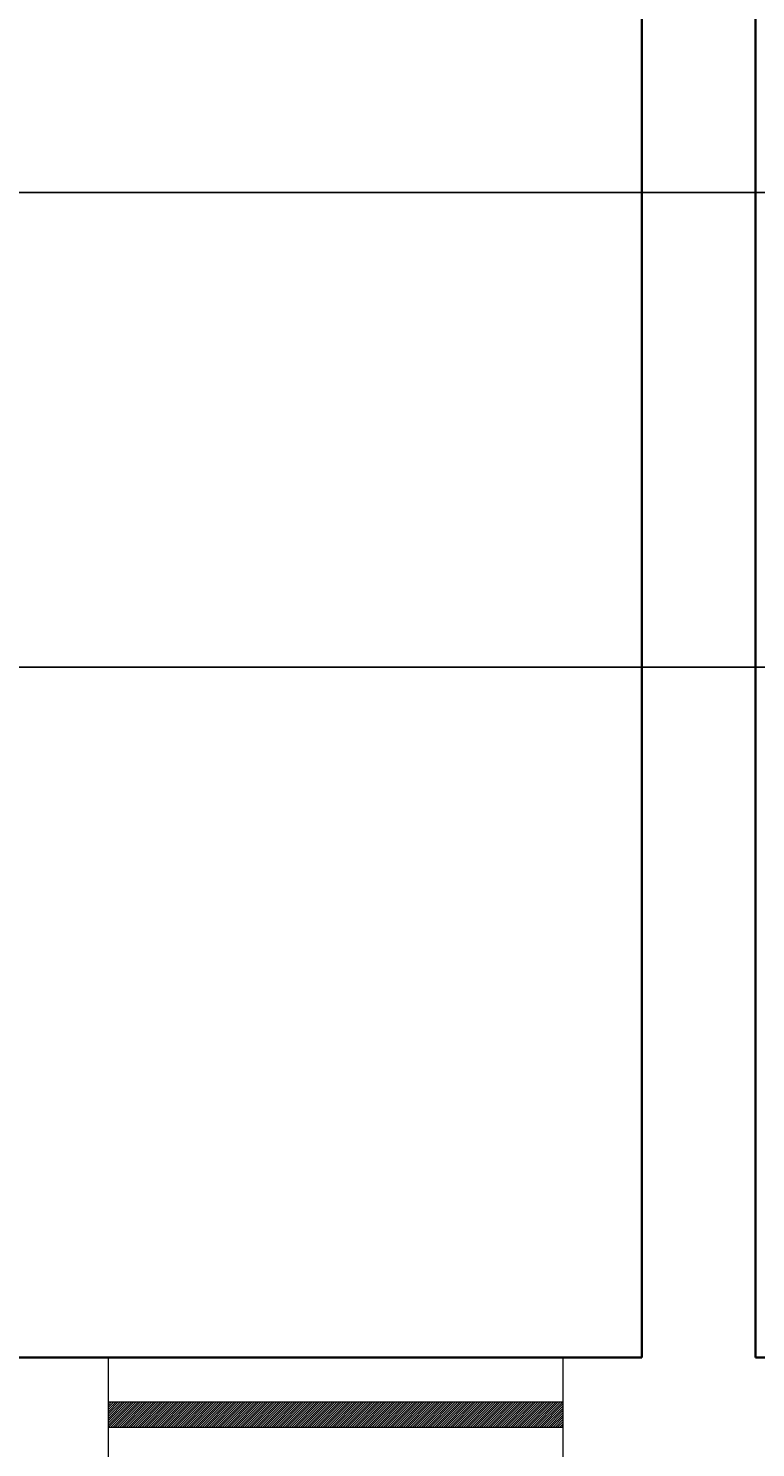
# Model space of a CAD drawing. Units: inches. Extents: x 318 to 927, y -1130 to 13.
# Tile 4 of 17: x 541 to 599, y -1041 to -929. Entities that reach past the tile are written whole.
import ezdxf

# ---------------------------------------------------------------- set-up
doc = ezdxf.new("R2010")
doc.units = ezdxf.units.IN
doc.header["$MEASUREMENT"] = 0
for name, color, linetype, lineweight in [('A-ANNO-DIMS', 1, 'Continuous', 18), ('A-GLAZ-PATT', 5, 'Continuous', 9), ('wall', 1, 'Continuous', 35), ('win', 5, 'Continuous', 18)]:
    doc.layers.add(name, color=color, linetype=linetype, lineweight=lineweight)
doc.styles.get("Standard").update_dxf_attribs({"font": 'arial.ttf'})
doc.dimstyles.get("Standard").update_dxf_attribs({"dimtxt": 0.18, "dimasz": 0.18, "dimexe": 0.18, "dimexo": 0.0625, "dimgap": 0.09, "dimtad": 0, "dimtih": 1, "dimtoh": 1, "dimdec": 1, "dimzin": 0, "dimdsep": 46, "dimlunit": 4, "dimtxsty": 'Standard', "dimcen": 0.09, "dimadec": 0, "dimazin": 0, "dimtfac": 1, "dimtdec": 1, "dimtofl": 0, "dimtmove": 0, "dimatfit": 3, "dimfxl": 1, "dimtolj": 1, "dimtzin": 0, "dimarcsym": 0})

# ---------------------------------------------------------------- blocks, each defined once
blk = doc.blocks.new('WIN-36IN')
for p, q in [((0, 36), (9, 36)), ((3.5, 36), (3.5, 0)), ((5.5, 36), (5.5, 0)), ((0, 0), (9, 0))]:
    blk.add_line(p, q)
blk = doc.blocks.new('*D55')
at = {"layer": 'A-ANNO-DIMS', "color": 0, "lineweight": -2, "transparency": 16777216}
for p, q in [((833.82, -941.75), (331.21, -941.75)), ((331.39, -941.93), (331.39, -960.35)), ((331.39, -979.13), (331.39, -960.71)), ((833.82, -979.31), (331.21, -979.31))]:
    blk.add_line(p, q, dxfattribs=at)
at = {"layer": 'A-ANNO-DIMS', "color": 0, "transparency": 16777216}
for points in [[(331.36, -941.93), (331.42, -941.93), (331.39, -941.75)], [(331.36, -979.13), (331.42, -979.13), (331.39, -979.31)]]:
    blk.add_solid(points, dxfattribs=at)
at = {"layer": 'Defpoints', "color": 0, "transparency": 16777216}
for p in [(833.89, -941.75), (331.39, -979.31), (833.89, -979.31)]:
    blk.add_point(p, dxfattribs=at)
at = {"layer": 'A-ANNO-DIMS', "color": 0, "transparency": 16777216, "insert": (331.39, -960.53), "char_height": 0.18, "attachment_point": 5}
blk.add_mtext('\\A1;3\'-1 1/2"', dxfattribs=at)

msp = doc.modelspace()

# ---------------------------------------------------------------- hatches: boundary and pattern name
at = {"layer": 'A-GLAZ-PATT'}
h = msp.add_hatch(dxfattribs=at)
h.set_pattern_fill('ANSI31', color=256)
h.paths.add_polyline_path([(787.43, -1037.41), (751.43, -1037.41), (751.43, -1039.41), (787.43, -1039.41)])
h.paths.add_polyline_path([(583.67, -1037.41), (547.67, -1037.41), (547.67, -1039.41), (583.67, -1039.41)])
h.paths.add_polyline_path([(394.39, -842.15), (392.39, -842.15), (392.39, -878.15), (394.39, -878.15)])
h.paths.add_polyline_path([(394.39, -788.96), (392.39, -788.96), (392.39, -812.96), (394.39, -812.96)])

# ---------------------------------------------------------------- linework, layer by layer
at = {"layer": 'wall'}
for p, q in [((589.89, -873.91), (589.89, -1033.91)), ((598.89, -873.91), (598.89, -1033.91)), ((397.89, -1033.91), (589.89, -1033.91)), ((598.89, -1033.91), (650.89, -1033.91))]:
    msp.add_line(p, q, dxfattribs=at)

# ---------------------------------------------------------------- block references
at = {"layer": 'win', "rotation": 89.99999999999967}
msp.add_blockref('WIN-36IN', (583.67, -1042.91), dxfattribs=at)

# ---------------------------------------------------------------- dimensions: what is measured, and where the dimension line sits
at = {"layer": 'A-ANNO-DIMS'}
dim = msp.add_linear_dim(base=(331.39, -979.31), p1=(833.89, -941.75), p2=(833.89, -979.31), angle=90, dimstyle='Standard', override={"dimdec": 1, "dimlfac": 1, "dimrnd": 0, "dimzin": 1, "dimdsep": 46, "dimlunit": 4, "dimfrac": 2}, dxfattribs=at)
dim.commit()
dim.dimension.update_dxf_attribs({"geometry": '*D55', "text_midpoint": (331.39, -960.53)})

doc.saveas('drawing.dxf')
